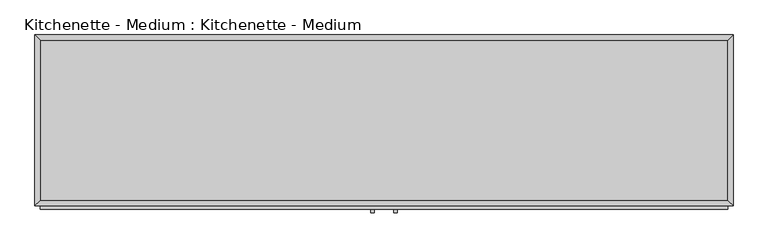
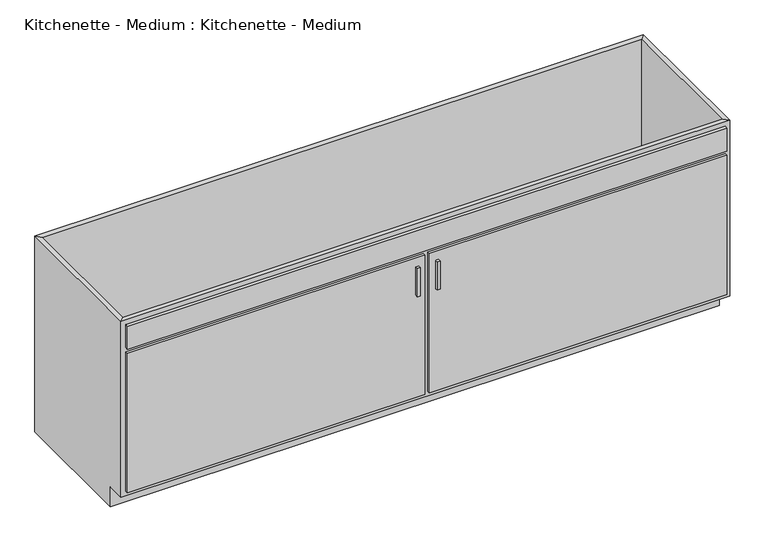
"""IFC4 building model written with IfcOpenShell, lengths in millimetres: proxy geometry, Kitchenette - Medium : Kitchenette - Medium."""

from ifc_helpers import new_model, si_unit, frame, origin, place, context, project, spatial, polyline, outline, extrude, faceted_brep, source, transform, mapped, element, save


def kitchenette_medium_kitchenette_medium_eaec4ed0(model_context):
    return source(origin(), model_context, "Body", "SolidModel", [
        extrude(outline(polyline([(1269.6877049, -19.05), (1269.6877049, -603.25), (-1232.2122951, -603.25), (-1232.2122951, -19.05), (1269.6877049, -19.05)])), frame((0.0, 0.0, 88.9), z_axis=(0.0, 0.0, 1.0), x_axis=(1.0, 0.0, 0.0)), (0.0, 0.0, 1.0), 19.05),
        extrude(outline(polyline([(-16.1872951, -647.7), (-28.8872951, -647.7), (-28.8872951, -635.0), (-16.1872951, -635.0), (-16.1872951, -647.7)])), frame((0.0, 0.0, 561.069895), z_axis=(0.0, 0.0, 1.0), x_axis=(1.0, 0.0, 0.0)), (0.0, 0.0, 1.0), 124.730105),
        extrude(outline(polyline([(66.3627049, -647.7), (53.6627049, -647.7), (53.6627049, -635.0), (66.3627049, -635.0), (66.3627049, -647.7)])), frame((0.0, 0.0, 561.069895), z_axis=(0.0, 0.0, 1.0), x_axis=(1.0, 0.0, 0.0)), (0.0, 0.0, 1.0), 124.730105),
        faceted_brep([(1269.6877049, -603.25, 863.6), (1269.6877049, -603.25, 88.9), (-1232.2122951, -603.25, 88.9), (-1232.2122951, -603.25, 863.6), (-1251.2622951, -622.3, 863.6), (1288.7377049, -622.3, 863.6), (-1251.2622951, -622.3, 88.9), (1288.7377049, -622.3, 88.9), (-1232.2122951, -546.1, 88.9), (-1232.2122951, -19.05, 88.9), (-1232.2122951, -19.05, 863.6), (-1251.2622951, 0.0, 863.6), (-1251.2622951, 0.0, 0.0), (-1251.2622951, -546.1, 0.0), (-1251.2622951, -546.1, 88.9), (1269.6877049, -19.05, 88.9), (1269.6877049, -19.05, 863.6), (1288.7377049, 0.0, 863.6), (1288.7377049, 0.0, 0.0), (1269.6877049, -546.1, 88.9), (1288.7377049, -546.1, 88.9), (1288.7377049, -546.1, 0.0)], [[[0, 1, 2, 3]], [[0, 3, 4, 5]], [[5, 4, 6, 7]], [[2, 1, 7, 6]], [[3, 2, 8, 9, 10]], [[4, 3, 10, 11]], [[6, 4, 11, 12, 13, 14]], [[2, 6, 14, 8]], [[10, 9, 15, 16]], [[11, 10, 16, 17]], [[12, 11, 17, 18]], [[1, 0, 16, 15, 19]], [[0, 5, 17, 16]], [[5, 7, 20, 21, 18, 17]], [[7, 1, 19, 20]], [[8, 19, 15, 9]], [[18, 21, 13, 12]], [[13, 21, 20, 19, 8, 14]]]),
        extrude(outline(polyline([(9.2127049, -635.0), (-1232.2122951, -635.0), (-1232.2122951, -622.3), (9.2127049, -622.3), (9.2127049, -635.0)])), frame((0.0, 0.0, 107.95), z_axis=(0.0, 0.0, 1.0), x_axis=(1.0, 0.0, 0.0)), (0.0, 0.0, 1.0), 615.95),
        extrude(outline(polyline([(1269.6877049, -635.0), (28.2627049, -635.0), (28.2627049, -622.3), (1269.6877049, -622.3), (1269.6877049, -635.0)])), frame((0.0, 0.0, 107.95), z_axis=(0.0, 0.0, 1.0), x_axis=(1.0, 0.0, 0.0)), (0.0, 0.0, 1.0), 615.95),
        extrude(outline(polyline([(1269.6877049, -635.0), (-1232.2122951, -635.0), (-1232.2122951, -622.3), (1269.6877049, -622.3), (1269.6877049, -635.0)])), frame((0.0, 0.0, 742.95), z_axis=(0.0, 0.0, 1.0), x_axis=(1.0, 0.0, 0.0)), (0.0, 0.0, 1.0), 101.6),
    ])


if __name__ == "__main__":
    model = new_model("IFC4")
    model_context = context("Model", 3, world=origin())
    ifc_project = project(units=[si_unit("LENGTHUNIT", "METRE", prefix="MILLI")], contexts=[model_context])
    site = spatial("IfcSite", under=ifc_project)
    building = spatial("IfcBuilding", under=site)
    placement = place(None, origin())
    kitchenette_medium_kitchenette_medium_shape = kitchenette_medium_kitchenette_medium_eaec4ed0(model_context)
    element("IfcBuildingElementProxy", 1, Name="Kitchenette - Medium : Kitchenette - Medium", ObjectType="Kitchenette - Medium : Kitchenette - Medium", at=placement, inside=building, context=model_context, shape_type="MappedRepresentation", body=[
        mapped(kitchenette_medium_kitchenette_medium_shape, transform((0.0, 0.0, 0.0), x_axis=(1.0, 0.0, 0.0), y_axis=(0.0, 1.0, 0.0), z_axis=(0.0, 0.0, 1.0))),
    ])
    save(model, "model.ifc")

# Revit data of these elements
# Type "Kitchenette - Medium : Kitchenette - Medium"
#   Assembly Code = "E1090400"
#   Sink Opening Depth = 1' - 2"
#   Sink Location To Wall = 0' - 6"
#   Sink Location = 3' - 4"
#   Counter Thickness = 0' - 1 1/2"
#   Counter Length = 16' - 8"
#   Cabinet Width = 8' - 4"
#   Cabinet Height = 2' - 10"
#   Cabinet Depth = 2' - 0 1/2"
#   Toe Depth = 0' - 3"
#   Toe Height = 0' - 3 1/2"
#   Cabinet Material = Cabinets
#   Door/Drawer Material = Cabinets
#   Handle Material = Cabinets - Handles
#   Default Elevation = 0
# Element 1 (IfcBuildingElementProxy, "Kitchenette - Medium : Kitchenette - Medium")
#   Materials on its faces: "Cabinets", "Cabinets - Handles"
# Materials
#   "Cabinets": colour RGB 249 249 249, transparency 0
#   "Cabinets - Handles": class "Metal", colour RGB 57 57 57, transparency 0
